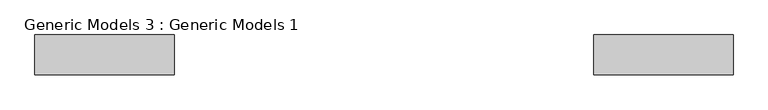
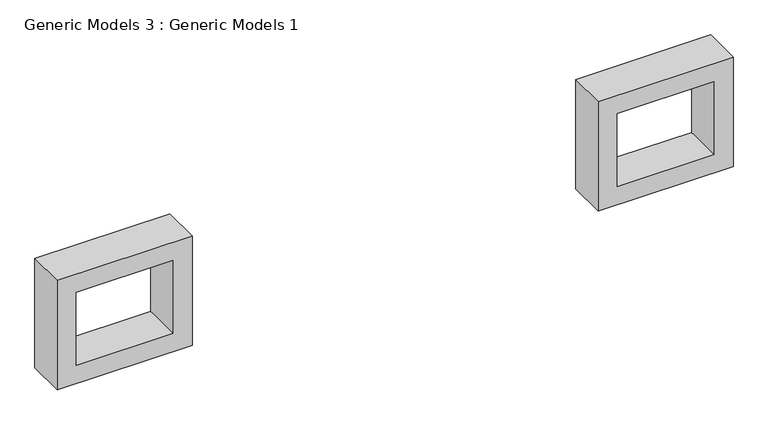
"""IFC4 building model written with IfcOpenShell, lengths in millimetres: proxy geometry, Generic Models 3 : Generic Models 1."""

from ifc_helpers import new_model, si_unit, frame, origin, place, context, project, spatial, polyline, outline, extrude, source, transform, mapped, element, save


def generic_models_3_generic_models_1_c81a4c1b(model_context):
    return source(origin(), model_context, "Body", "SweptSolid", [
        extrude(outline(polyline([(12039.6, -3915.3833787), (12039.6, -6048.9833787), (10210.8, -6048.9833787), (10210.8, -3915.3833787), (12039.6, -3915.3833787)]), holes=[polyline([(11734.8, -4220.1833787), (10515.6, -4220.1833787), (10515.6, -5744.1833787), (11734.8, -5744.1833787), (11734.8, -4220.1833787)])]), frame((0.0, -10658.540066, 0.0), z_axis=(0.0, 1.0, 0.0), x_axis=(0.0, 0.0, 1.0)), (0.0, 0.0, 1.0), 609.6),
        extrude(outline(polyline([(12039.6, 4631.7166213), (12039.6, 2498.1166213), (10210.8, 2498.1166213), (10210.8, 4631.7166213), (12039.6, 4631.7166213)]), holes=[polyline([(11734.8, 4326.9166213), (10515.6, 4326.9166213), (10515.6, 2802.9166213), (11734.8, 2802.9166213), (11734.8, 4326.9166213)])]), frame((0.0, -10658.540066, 0.0), z_axis=(0.0, 1.0, 0.0), x_axis=(0.0, 0.0, 1.0)), (0.0, 0.0, 1.0), 609.6),
    ])


if __name__ == "__main__":
    model = new_model("IFC4")
    model_context = context("Model", 3, world=origin())
    ifc_project = project(units=[si_unit("LENGTHUNIT", "METRE", prefix="MILLI")], contexts=[model_context])
    site = spatial("IfcSite", under=ifc_project)
    building = spatial("IfcBuilding", under=site)
    placement = place(None, origin())
    generic_models_3_generic_models_1_shape = generic_models_3_generic_models_1_c81a4c1b(model_context)
    element("IfcBuildingElementProxy", 1, Name="Generic Models 3 : Generic Models 1", ObjectType="Generic Models 3 : Generic Models 1", at=placement, inside=building, context=model_context, shape_type="MappedRepresentation", body=[
        mapped(generic_models_3_generic_models_1_shape, transform((0.0, 0.0, 0.0), x_axis=(1.0, 0.0, 0.0), y_axis=(0.0, 1.0, 0.0), z_axis=(0.0, 0.0, 1.0))),
    ])
    save(model, "model.ifc")

# Revit data of these elements
# Element 1 (IfcBuildingElementProxy, "Generic Models 3 : Generic Models 1")
#   Materials on its faces: "grey"
# Materials
#   "grey": class "Generic", colour RGB 33 34 34, transparency 0, Cost = 0
